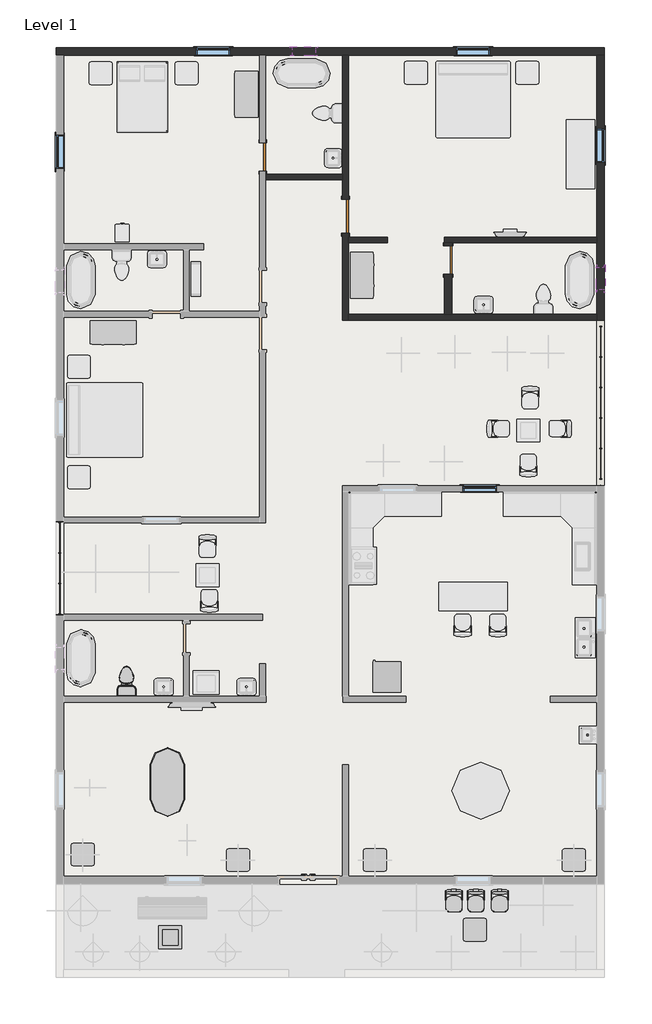
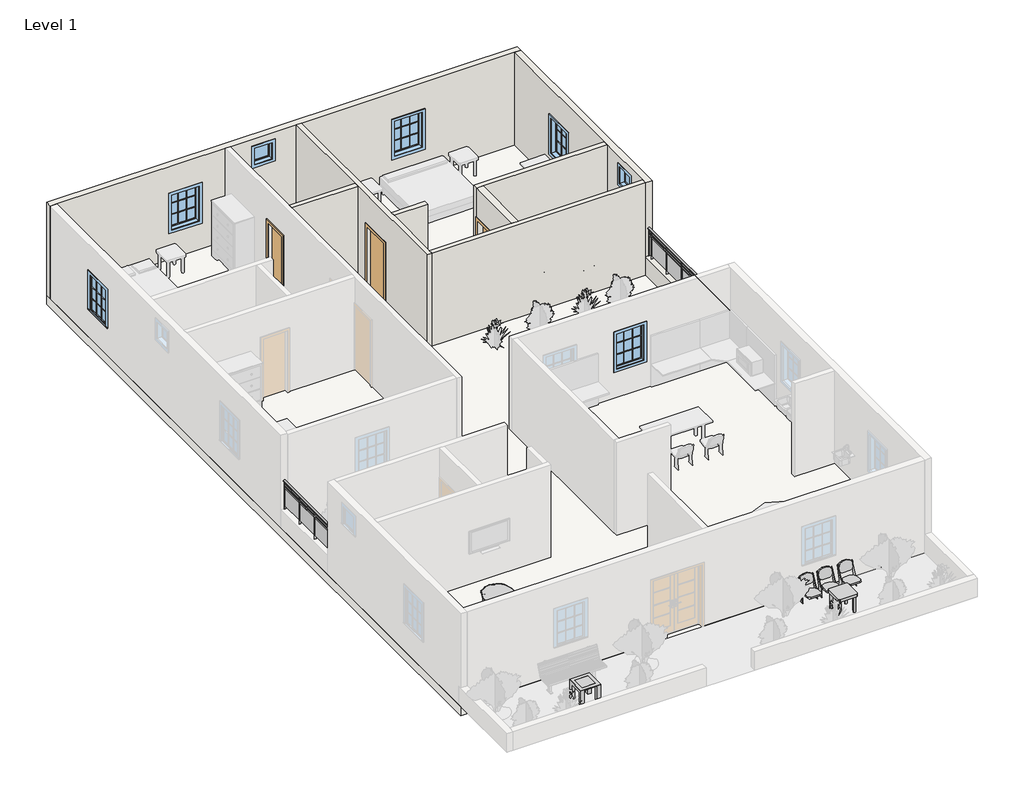
# One storey, part 2 of 3: 10 furniture elements, 9 walls, 7 windows, 3 doors, 2 flow terminals, 2 railings, 1 slab.
"""IFC4 building model written with IfcOpenShell, lengths in millimetres."""

from ifc_helpers import new_model, si_unit, point, frame, origin, origin_with_axes, place, context, project, spatial, polyline, ellipse_curve, trimmed, outline, extrude, faceted_brep, transform, mapped, element, save
from ifc_brep_helpers import plane_surface, extruded_surface, advanced_brep
from components import door_059fdd7e, door_53b1b562, door_193fcfdc, flow_terminal_accce45a, toilet_domestic_3d_toilet_domestic_3d_f7549cf7, toilet_domestic_3d_toilet_domestic_3d_183bbd19, furniture_3d1d9cbc, furniture_b5c51a22, furniture_2c34a4f9, furniture_31d08a24, window_29c06734, window_5c190c7e, window_e41d21a6

model = new_model("IFC4")

# Units and contexts
model_context = context("Model", 3, world=origin())
ifc_project = project(units=[si_unit("LENGTHUNIT", "METRE", prefix="MILLI")], contexts=[model_context])

# Site, building, storey
site = spatial("IfcSite", under=ifc_project)
building = spatial("IfcBuilding", under=site)
storey = spatial("IfcBuildingStorey", under=building, Name="Level 1", Elevation=0.0)

# Doors
placement = place(None, origin())
door_shape = door_059fdd7e(model_context)
element("IfcDoor", 1, ObjectType="Single-Flush : 30\" x 80\"", at=placement, inside=storey, context=model_context, shape_type="MappedRepresentation", body=[
    mapped(door_shape, transform((-9555.9446525, 9738.3002171, 0.0), x_axis=(0.0, -1.0, 0.0), y_axis=(1.0, 0.0, 0.0), z_axis=(0.0, 0.0, 1.0))),
])
door_2_shape = door_53b1b562(model_context)
element("IfcDoor", 2, ObjectType="Single-Flush : 30\" x 80\"", at=placement, inside=storey, context=model_context, shape_type="MappedRepresentation", body=[
    mapped(door_2_shape, transform((-4602.9446525, 6995.1002171, 0.0), x_axis=(0.0, 1.0, 0.0), y_axis=(-1.0, 0.0, 0.0), z_axis=(0.0, 0.0, 1.0))),
])
door_3_shape = door_193fcfdc(model_context)
element("IfcDoor", 3, ObjectType="Single-Flush : 36\" x 80\"", at=placement, inside=storey, context=model_context, shape_type="MappedRepresentation", body=[
    mapped(door_3_shape, transform((-7346.1446525, 8163.5002171, 0.0), x_axis=(0.0, -1.0, 0.0), y_axis=(1.0, 0.0, 0.0), z_axis=(0.0, 0.0, 1.0))),
])

# Flow terminals
flow_terminal_shape = flow_terminal_accce45a(model_context)
element("IfcFlowTerminal", 4, ObjectType="Floor Drain - Round : 5\" Strainer - 2\" Drain", at=placement, inside=storey, context=model_context, shape_type="MappedRepresentation", body=[
    mapped(flow_terminal_shape, transform((-13721.5446525, -4257.0997829, 0.0), x_axis=(1.0, 0.0, 0.0), y_axis=(0.0, 1.0, 0.0), z_axis=(0.0, 0.0, 1.0))),
])
toilet_domestic_3d_toilet_domestic_3d_shape = toilet_domestic_3d_toilet_domestic_3d_f7549cf7(model_context)
toilet_domestic_3d_toilet_domestic_3d_2_shape = toilet_domestic_3d_toilet_domestic_3d_183bbd19(model_context)
element("IfcFlowTerminal", 5, ObjectType="Toilet-Domestic-3D : Toilet-Domestic-3D", at=placement, inside=storey, context=model_context, shape_type="MappedRepresentation", body=[
    mapped(toilet_domestic_3d_toilet_domestic_3d_shape, transform((-13188.1446525, -4143.4037556, 0.0), x_axis=(-1.0000000000000004, 0.0, 0.0), y_axis=(0.0, -1.0000000000000004, 0.0), z_axis=(0.0, 0.0, 1.0))),
    mapped(toilet_domestic_3d_toilet_domestic_3d_2_shape, transform((-13188.1446525, -4143.4037556, 0.0), x_axis=(-1.0000000000000004, 0.0, 0.0), y_axis=(0.0, -1.0000000000000004, 0.0), z_axis=(0.0, 0.0, 1.0))),
])

# Furniture
furniture_shape = furniture_3d1d9cbc(model_context)
element("IfcFurniture", 6, ObjectType="Seating-Auditorium : 18\" x 24\" x 30\"", at=placement, inside=storey, context=model_context, shape_type="MappedRepresentation", body=[
    mapped(furniture_shape, transform((-4289.8167836, -9883.8243731, 0.0), x_axis=(-1.0000000000000004, 0.0, 0.0), y_axis=(0.0, -1.0000000000000004, 0.0), z_axis=(0.0, 0.0, 1.0))),
])
element("IfcFurniture", 7, ObjectType="Seating-Auditorium : 18\" x 24\" x 30\"", at=placement, inside=storey, context=model_context, shape_type="MappedRepresentation", body=[
    mapped(furniture_shape, transform((-3705.6167836, -9883.8243731, 0.0), x_axis=(-1.0000000000000004, 0.0, 0.0), y_axis=(0.0, -1.0000000000000004, 0.0), z_axis=(0.0, 0.0, 1.0))),
])
element("IfcFurniture", 8, ObjectType="Seating-Auditorium : 18\" x 24\" x 30\"", at=placement, inside=storey, context=model_context, shape_type="MappedRepresentation", body=[
    mapped(furniture_shape, transform((-3070.6167836, -9883.8243731, 0.0), x_axis=(-1.0000000000000004, 0.0, 0.0), y_axis=(0.0, -1.0000000000000004, 0.0), z_axis=(0.0, 0.0, 1.0))),
])
furniture_2_shape = furniture_b5c51a22(model_context)
element("IfcFurniture", 9, ObjectType="Table-Coffee : 24\" x 24\" x 24\"", at=placement, inside=storey, context=model_context, shape_type="MappedRepresentation", body=[
    mapped(furniture_2_shape, transform((-12038.0104192, -11159.5108607, 0.0), x_axis=(1.0, 0.0, 0.0), y_axis=(0.0, 1.0, 0.0), z_axis=(0.0, 0.0, 1.0))),
])
furniture_3_shape = furniture_2c34a4f9(model_context)
element("IfcFurniture", 10, ObjectType="Table-Dining Oval : 36\" x 72\"", at=placement, inside=storey, context=model_context, shape_type="MappedRepresentation", body=[
    mapped(furniture_3_shape, transform((-12454.0430131, -6522.2801108, 0.0), x_axis=(0.0, 1.0000000000000002, 0.0), y_axis=(-1.0000000000000002, 0.0, 0.0), z_axis=(0.0, 0.0, 1.0))),
])
furniture_4_shape = furniture_31d08a24(model_context)
element("IfcFurniture", 11, ObjectType="Table-End : 24\" x 24\"", at=placement, inside=storey, context=model_context, shape_type="MappedRepresentation", body=[
    mapped(furniture_4_shape, transform((-14665.0782828, -9006.8997829, 0.0), x_axis=(1.0, 0.0, 0.0), y_axis=(0.0, 1.0, 0.0), z_axis=(0.0, 0.0, 1.0))),
])
element("IfcFurniture", 12, ObjectType="Table-End : 24\" x 24\"", at=placement, inside=storey, context=model_context, shape_type="MappedRepresentation", body=[
    mapped(furniture_4_shape, transform((-10524.8782828, -9152.9497829, 0.0), x_axis=(1.0, 0.0, 0.0), y_axis=(0.0, 1.0, 0.0), z_axis=(0.0, 0.0, 1.0))),
])
element("IfcFurniture", 13, ObjectType="Table-End : 24\" x 24\"", at=placement, inside=storey, context=model_context, shape_type="MappedRepresentation", body=[
    mapped(furniture_4_shape, transform((-6867.2782828, -9152.9497829, 0.0), x_axis=(1.0, 0.0, 0.0), y_axis=(0.0, 1.0, 0.0), z_axis=(0.0, 0.0, 1.0))),
])
element("IfcFurniture", 14, ObjectType="Table-End : 24\" x 24\"", at=placement, inside=storey, context=model_context, shape_type="MappedRepresentation", body=[
    mapped(furniture_4_shape, transform((-1558.6782828, -9152.9497829, 0.0), x_axis=(1.0, 0.0, 0.0), y_axis=(0.0, 1.0, 0.0), z_axis=(0.0, 0.0, 1.0))),
])
element("IfcFurniture", 15, ObjectType="Table-End : 24\" x 24\"", at=placement, inside=storey, context=model_context, shape_type="MappedRepresentation", body=[
    mapped(furniture_4_shape, transform((-4200.2782828, -11013.4997829, 0.0), x_axis=(1.0, 0.0, 0.0), y_axis=(0.0, 1.0, 0.0), z_axis=(0.0, 0.0, 1.0))),
])

# Railings
element("IfcRailing", 16, ObjectType="Glass Panel - Bottom Fill", at=placement, inside=storey, context=model_context, shape_type="SolidModel", body=[
    advanced_brep(
    [(-14928.0446525, 35.5002171, 1524.0), (-15004.2446525, 35.5002171, 1524.0), (-14928.0446525, -2479.0997829, 1524.0), (-15004.2446525, -2479.0997829, 1524.0)],
    [
        (0, 1, ellipse_curve(frame((-14966.1446525, 35.5002171, 1524.0), z_axis=(0.0, 1.0, 0.0), x_axis=(-1.0, 0.0, 0.0)), 38.1, 28.575)),
        (1, 0, ellipse_curve(frame((-14966.1446525, 35.5002171, 1524.0), z_axis=(0.0, 1.0, 0.0), x_axis=(-1.0, 0.0, 0.0)), 38.1, 28.575)),
        (2, 3, ellipse_curve(frame((-14966.1446525, -2479.0997829, 1524.0), z_axis=(0.0, -1.0, 0.0), x_axis=(-1.0, 0.0, 0.0)), 38.1, 28.575)),
        (3, 2, ellipse_curve(frame((-14966.1446525, -2479.0997829, 1524.0), z_axis=(0.0, -1.0, 0.0), x_axis=(-1.0, 0.0, 0.0)), 38.1, 28.575)),
        (0, 2),
        (3, 1),
    ],
    [
        plane_surface(frame((-14966.1446525, 35.5002171, 1524.0), z_axis=(0.0, 1.0, 0.0), x_axis=(0.0, 0.0, -1.0))),
        plane_surface(frame((-14966.1446525, -2479.0997829, 1524.0), z_axis=(0.0, -1.0, 0.0), x_axis=(0.0, 0.0, -1.0))),
        extruded_surface(trimmed(ellipse_curve(frame((-14966.1446525, -2479.0997829, 1524.0), z_axis=(0.0, 1.0, 0.0), x_axis=(-1.0, 0.0, 0.0)), 38.1, 28.575), [point((-14928.0446525, -2479.0997829, 1524.0))], [point((-15004.2446525, -2479.0997829, 1524.0))], True, "CARTESIAN"), (0.0, 2514.6, 0.0), 2514.6),
        extruded_surface(trimmed(ellipse_curve(frame((-14966.1446525, -2479.0997829, 1524.0), z_axis=(0.0, 1.0, 0.0), x_axis=(-1.0, 0.0, 0.0)), 38.1, 28.575), [point((-15004.2446525, -2479.0997829, 1524.0))], [point((-14928.0446525, -2479.0997829, 1524.0))], True, "CARTESIAN"), (0.0, 2514.6, 0.0), 2514.6),
    ],
    [
        (0, [[1, 2]]),
        (1, [[3, 4]]),
        (2, [[-1, 5, -4, 6]]),
        (3, [[-2, -6, -3, -5]]),
    ],
),
    extrude(outline(polyline([(-14978.8446525, 35.5002171), (-14953.4446525, 35.5002171), (-14953.4446525, -2479.0997829), (-14978.8446525, -2479.0997829), (-14978.8446525, 35.5002171)])), frame((0.0, 0.0, 1409.7), z_axis=(0.0, 0.0, 1.0), x_axis=(1.0, 0.0, 0.0)), (0.0, 0.0, 1.0), 25.4),
    extrude(outline(polyline([(-14978.8446525, 35.5002171), (-14953.4446525, 35.5002171), (-14953.4446525, -2479.0997829), (-14978.8446525, -2479.0997829), (-14978.8446525, 35.5002171)])), frame((0.0, 0.0, 1308.1), z_axis=(0.0, 0.0, 1.0), x_axis=(1.0, 0.0, 0.0)), (0.0, 0.0, 1.0), 25.4),
    extrude(outline(polyline([(-14991.5446525, -2434.6497829), (-14940.7446525, -2434.6497829), (-14940.7446525, -2447.3497829), (-14991.5446525, -2447.3497829), (-14991.5446525, -2434.6497829)])), frame((0.0, 0.0, 609.6), z_axis=(0.0, 0.0, 1.0), x_axis=(1.0, 0.0, 0.0)), (0.0, 0.0, 1.0), 885.6788223),
    extrude(outline(polyline([(-14959.6094955, -1628.1997829), (-14959.6094955, -2440.9997829), (-14965.9594955, -2440.9997829), (-14965.9594955, -1628.1997829), (-14959.6094955, -1628.1997829)])), frame((0.0, 0.0, 711.2), z_axis=(0.0, 0.0, 1.0), x_axis=(1.0, 0.0, 0.0)), (0.0, 0.0, 1.0), 596.9),
    extrude(outline(polyline([(-14991.5446525, -1621.8497829), (-14940.7446525, -1621.8497829), (-14940.7446525, -1634.5497829), (-14991.5446525, -1634.5497829), (-14991.5446525, -1621.8497829)])), frame((0.0, 0.0, 609.6), z_axis=(0.0, 0.0, 1.0), x_axis=(1.0, 0.0, 0.0)), (0.0, 0.0, 1.0), 885.6788223),
    extrude(outline(polyline([(-14959.6094955, -815.3997829), (-14959.6094955, -1628.1997829), (-14965.9594955, -1628.1997829), (-14965.9594955, -815.3997829), (-14959.6094955, -815.3997829)])), frame((0.0, 0.0, 711.2), z_axis=(0.0, 0.0, 1.0), x_axis=(1.0, 0.0, 0.0)), (0.0, 0.0, 1.0), 596.9),
    extrude(outline(polyline([(-14991.5446525, -809.0497829), (-14940.7446525, -809.0497829), (-14940.7446525, -821.7497829), (-14991.5446525, -821.7497829), (-14991.5446525, -809.0497829)])), frame((0.0, 0.0, 609.6), z_axis=(0.0, 0.0, 1.0), x_axis=(1.0, 0.0, 0.0)), (0.0, 0.0, 1.0), 885.6788223),
    extrude(outline(polyline([(-14959.6094955, -2.5997829), (-14959.6094955, -815.3997829), (-14965.9594955, -815.3997829), (-14965.9594955, -2.5997829), (-14959.6094955, -2.5997829)])), frame((0.0, 0.0, 711.2), z_axis=(0.0, 0.0, 1.0), x_axis=(1.0, 0.0, 0.0)), (0.0, 0.0, 1.0), 596.9),
    extrude(outline(polyline([(-14991.5446525, 3.7502171), (-14940.7446525, 3.7502171), (-14940.7446525, -8.9497829), (-14991.5446525, -8.9497829), (-14991.5446525, 3.7502171)])), frame((0.0, 0.0, 609.6), z_axis=(0.0, 0.0, 1.0), x_axis=(1.0, 0.0, 0.0)), (0.0, 0.0, 1.0), 885.6788223),
    extrude(outline(polyline([(-14975.6696525, -2466.3997829), (-14956.6196525, -2466.3997829), (-14956.6196525, -2485.4497829), (-14975.6696525, -2485.4497829), (-14975.6696525, -2466.3997829)])), frame((0.0, 0.0, 609.6), z_axis=(0.0, 0.0, 1.0), x_axis=(1.0, 0.0, 0.0)), (0.0, 0.0, 1.0), 885.6788223),
    extrude(outline(polyline([(-14975.6696525, 41.8502171), (-14956.6196525, 41.8502171), (-14956.6196525, 22.8002171), (-14975.6696525, 22.8002171), (-14975.6696525, 41.8502171)])), frame((0.0, 0.0, 609.6), z_axis=(0.0, 0.0, 1.0), x_axis=(1.0, 0.0, 0.0)), (0.0, 0.0, 1.0), 885.6788223),
])
element("IfcRailing", 17, ObjectType="Glass Panel - Bottom Fill", at=placement, inside=storey, context=model_context, shape_type="SolidModel", body=[
    advanced_brep(
    [(-500.8446525, 5394.9002171, 1524.0), (-577.0446525, 5394.9002171, 1524.0), (-500.8446525, 975.3002171, 1524.0), (-577.0446525, 975.3002171, 1524.0)],
    [
        (0, 1, ellipse_curve(frame((-538.9446525, 5394.9002171, 1524.0), z_axis=(0.0, 1.0, 0.0), x_axis=(-1.0, 0.0, 0.0)), 38.1, 28.575)),
        (1, 0, ellipse_curve(frame((-538.9446525, 5394.9002171, 1524.0), z_axis=(0.0, 1.0, 0.0), x_axis=(-1.0, 0.0, 0.0)), 38.1, 28.575)),
        (2, 3, ellipse_curve(frame((-538.9446525, 975.3002171, 1524.0), z_axis=(0.0, -1.0, 0.0), x_axis=(-1.0, 0.0, 0.0)), 38.1, 28.575)),
        (3, 2, ellipse_curve(frame((-538.9446525, 975.3002171, 1524.0), z_axis=(0.0, -1.0, 0.0), x_axis=(-1.0, 0.0, 0.0)), 38.1, 28.575)),
        (0, 2),
        (3, 1),
    ],
    [
        plane_surface(frame((-538.9446525, 5394.9002171, 1524.0), z_axis=(0.0, 1.0, 0.0), x_axis=(0.0, 0.0, -1.0))),
        plane_surface(frame((-538.9446525, 975.3002171, 1524.0), z_axis=(0.0, -1.0, 0.0), x_axis=(0.0, 0.0, -1.0))),
        extruded_surface(trimmed(ellipse_curve(frame((-538.9446525, 975.3002171, 1524.0), z_axis=(0.0, 1.0, 0.0), x_axis=(-1.0, 0.0, 0.0)), 38.1, 28.575), [point((-500.8446525, 975.3002171, 1524.0))], [point((-577.0446525, 975.3002171, 1524.0))], True, "CARTESIAN"), (0.0, 4419.6, 0.0), 4419.6),
        extruded_surface(trimmed(ellipse_curve(frame((-538.9446525, 975.3002171, 1524.0), z_axis=(0.0, 1.0, 0.0), x_axis=(-1.0, 0.0, 0.0)), 38.1, 28.575), [point((-577.0446525, 975.3002171, 1524.0))], [point((-500.8446525, 975.3002171, 1524.0))], True, "CARTESIAN"), (0.0, 4419.6, 0.0), 4419.6),
    ],
    [
        (0, [[1, 2]]),
        (1, [[3, 4]]),
        (2, [[-1, 5, -4, 6]]),
        (3, [[-2, -6, -3, -5]]),
    ],
),
    extrude(outline(polyline([(-551.6446525, 5394.9002171), (-526.2446525, 5394.9002171), (-526.2446525, 975.3002171), (-551.6446525, 975.3002171), (-551.6446525, 5394.9002171)])), frame((0.0, 0.0, 1409.7), z_axis=(0.0, 0.0, 1.0), x_axis=(1.0, 0.0, 0.0)), (0.0, 0.0, 1.0), 25.4),
    extrude(outline(polyline([(-551.6446525, 5394.9002171), (-526.2446525, 5394.9002171), (-526.2446525, 975.3002171), (-551.6446525, 975.3002171), (-551.6446525, 5394.9002171)])), frame((0.0, 0.0, 1308.1), z_axis=(0.0, 0.0, 1.0), x_axis=(1.0, 0.0, 0.0)), (0.0, 0.0, 1.0), 25.4),
    extrude(outline(polyline([(-564.3446525, 1159.4502171), (-513.5446525, 1159.4502171), (-513.5446525, 1146.7502171), (-564.3446525, 1146.7502171), (-564.3446525, 1159.4502171)])), frame((0.0, 0.0, 609.6), z_axis=(0.0, 0.0, 1.0), x_axis=(1.0, 0.0, 0.0)), (0.0, 0.0, 1.0), 885.6788223),
    extrude(outline(polyline([(-532.4094955, 1965.9002171), (-532.4094955, 1153.1002171), (-538.7594955, 1153.1002171), (-538.7594955, 1965.9002171), (-532.4094955, 1965.9002171)])), frame((0.0, 0.0, 711.2), z_axis=(0.0, 0.0, 1.0), x_axis=(1.0, 0.0, 0.0)), (0.0, 0.0, 1.0), 596.9),
    extrude(outline(polyline([(-564.3446525, 1972.2502171), (-513.5446525, 1972.2502171), (-513.5446525, 1959.5502171), (-564.3446525, 1959.5502171), (-564.3446525, 1972.2502171)])), frame((0.0, 0.0, 609.6), z_axis=(0.0, 0.0, 1.0), x_axis=(1.0, 0.0, 0.0)), (0.0, 0.0, 1.0), 885.6788223),
    extrude(outline(polyline([(-532.4094955, 2778.7002171), (-532.4094955, 1965.9002171), (-538.7594955, 1965.9002171), (-538.7594955, 2778.7002171), (-532.4094955, 2778.7002171)])), frame((0.0, 0.0, 711.2), z_axis=(0.0, 0.0, 1.0), x_axis=(1.0, 0.0, 0.0)), (0.0, 0.0, 1.0), 596.9),
    extrude(outline(polyline([(-564.3446525, 2785.0502171), (-513.5446525, 2785.0502171), (-513.5446525, 2772.3502171), (-564.3446525, 2772.3502171), (-564.3446525, 2785.0502171)])), frame((0.0, 0.0, 609.6), z_axis=(0.0, 0.0, 1.0), x_axis=(1.0, 0.0, 0.0)), (0.0, 0.0, 1.0), 885.6788223),
    extrude(outline(polyline([(-532.4094955, 3591.5002171), (-532.4094955, 2778.7002171), (-538.7594955, 2778.7002171), (-538.7594955, 3591.5002171), (-532.4094955, 3591.5002171)])), frame((0.0, 0.0, 711.2), z_axis=(0.0, 0.0, 1.0), x_axis=(1.0, 0.0, 0.0)), (0.0, 0.0, 1.0), 596.9),
    extrude(outline(polyline([(-564.3446525, 3597.8502171), (-513.5446525, 3597.8502171), (-513.5446525, 3585.1502171), (-564.3446525, 3585.1502171), (-564.3446525, 3597.8502171)])), frame((0.0, 0.0, 609.6), z_axis=(0.0, 0.0, 1.0), x_axis=(1.0, 0.0, 0.0)), (0.0, 0.0, 1.0), 885.6788223),
    extrude(outline(polyline([(-532.4094955, 4404.3002171), (-532.4094955, 3591.5002171), (-538.7594955, 3591.5002171), (-538.7594955, 4404.3002171), (-532.4094955, 4404.3002171)])), frame((0.0, 0.0, 711.2), z_axis=(0.0, 0.0, 1.0), x_axis=(1.0, 0.0, 0.0)), (0.0, 0.0, 1.0), 596.9),
    extrude(outline(polyline([(-564.3446525, 4410.6502171), (-513.5446525, 4410.6502171), (-513.5446525, 4397.9502171), (-564.3446525, 4397.9502171), (-564.3446525, 4410.6502171)])), frame((0.0, 0.0, 609.6), z_axis=(0.0, 0.0, 1.0), x_axis=(1.0, 0.0, 0.0)), (0.0, 0.0, 1.0), 885.6788223),
    extrude(outline(polyline([(-532.4094955, 5217.1002171), (-532.4094955, 4404.3002171), (-538.7594955, 4404.3002171), (-538.7594955, 5217.1002171), (-532.4094955, 5217.1002171)])), frame((0.0, 0.0, 711.2), z_axis=(0.0, 0.0, 1.0), x_axis=(1.0, 0.0, 0.0)), (0.0, 0.0, 1.0), 596.9),
    extrude(outline(polyline([(-564.3446525, 5223.4502171), (-513.5446525, 5223.4502171), (-513.5446525, 5210.7502171), (-564.3446525, 5210.7502171), (-564.3446525, 5223.4502171)])), frame((0.0, 0.0, 609.6), z_axis=(0.0, 0.0, 1.0), x_axis=(1.0, 0.0, 0.0)), (0.0, 0.0, 1.0), 885.6788223),
    extrude(outline(polyline([(-548.4696525, 988.0002171), (-529.4196525, 988.0002171), (-529.4196525, 968.9502171), (-548.4696525, 968.9502171), (-548.4696525, 988.0002171)])), frame((0.0, 0.0, 609.6), z_axis=(0.0, 0.0, 1.0), x_axis=(1.0, 0.0, 0.0)), (0.0, 0.0, 1.0), 885.6788223),
    extrude(outline(polyline([(-548.4696525, 5401.2502171), (-529.4196525, 5401.2502171), (-529.4196525, 5382.2002171), (-548.4696525, 5382.2002171), (-548.4696525, 5401.2502171)])), frame((0.0, 0.0, 609.6), z_axis=(0.0, 0.0, 1.0), x_axis=(1.0, 0.0, 0.0)), (0.0, 0.0, 1.0), 885.6788223),
])

# Slab
element("IfcSlab", 18, ObjectType="Generic - 12\"", at=placement, inside=storey, context=model_context, shape_type="SweptSolid", body=[
    extrude(outline(polyline([(-437.3446525, 12659.3002171), (-437.3446525, -9641.8997829), (-15067.7446525, -9641.8997829), (-15067.7446525, 12659.3002171), (-437.3446525, 12659.3002171)])), frame((0.0, 0.0, -304.8), z_axis=(0.0, 0.0, 1.0), x_axis=(1.0, 0.0, 0.0)), (0.0, 0.0, 1.0), 304.8),
])

# Walls
element("IfcWall", 19, ObjectType="Generic - 2'", at=placement, inside=storey, context=model_context, shape_type="Brep", body=[
    faceted_brep([(-640.5446525, 5471.1002171, 0.0), (-640.5446525, 5394.9002171, 0.0), (-640.5446525, 975.3002171, 0.0), (-640.5446525, 899.1002171, 0.0), (-640.5446525, 899.1002171, 609.6), (-640.5446525, 5471.1002171, 609.6), (-437.3446525, 5471.1002171, 0.0), (-437.3446525, 5471.1002171, 609.6), (-437.3446525, 899.1002171, 609.6), (-437.3446525, 899.1002171, 0.0)], [[[0, 1, 2, 3, 4, 5]], [[6, 7, 8, 9]], [[3, 2, 1, 0, 6, 9]], [[4, 3, 9, 8]], [[5, 4, 8, 7]], [[0, 5, 7, 6]]]),
])
element("IfcWall", 20, ObjectType="Generic - 8\"", at=placement, inside=storey, context=model_context, shape_type="Brep", body=[
    faceted_brep([(-15067.7446525, 12456.1002171, 0.0), (-14864.5446525, 12456.1002171, 0.0), (-9632.1446525, 12456.1002171, 0.0), (-9479.7446525, 12456.1002171, 0.0), (-7422.3446525, 12456.1002171, 0.0), (-7269.9446525, 12456.1002171, 0.0), (-640.5446525, 12456.1002171, 0.0), (-437.3446525, 12456.1002171, 0.0), (-437.3446525, 12456.1002171, 3048.0), (-640.5446525, 12456.1002171, 3048.0), (-7269.9446525, 12456.1002171, 3048.0), (-7422.3446525, 12456.1002171, 3048.0), (-9479.7446525, 12456.1002171, 3048.0), (-9632.1446525, 12456.1002171, 3048.0), (-14864.5446525, 12456.1002171, 3048.0), (-15067.7446525, 12456.1002171, 3048.0), (-3485.3446525, 12456.1002171, 2133.6), (-3485.3446525, 12456.1002171, 914.4), (-4399.7446525, 12456.1002171, 914.4), (-4399.7446525, 12456.1002171, 2133.6), (-10419.5446525, 12456.1002171, 2133.6), (-10419.5446525, 12456.1002171, 914.4), (-11333.9446525, 12456.1002171, 914.4), (-11333.9446525, 12456.1002171, 2133.6), (-8146.2446525, 12456.1002171, 2768.6), (-8146.2446525, 12456.1002171, 2159.0), (-8755.8446525, 12456.1002171, 2159.0), (-8755.8446525, 12456.1002171, 2768.6), (-15067.7446525, 12659.3002171, 0.0), (-15067.7446525, 12659.3002171, 3048.0), (-437.3446525, 12659.3002171, 3048.0), (-437.3446525, 12659.3002171, 0.0), (-3485.3446525, 12659.3002171, 2133.6), (-4399.7446525, 12659.3002171, 2133.6), (-4399.7446525, 12659.3002171, 914.4), (-3485.3446525, 12659.3002171, 914.4), (-10419.5446525, 12659.3002171, 2133.6), (-11333.9446525, 12659.3002171, 2133.6), (-11333.9446525, 12659.3002171, 914.4), (-10419.5446525, 12659.3002171, 914.4), (-8146.2446525, 12659.3002171, 2768.6), (-8755.8446525, 12659.3002171, 2768.6), (-8755.8446525, 12659.3002171, 2159.0), (-8146.2446525, 12659.3002171, 2159.0)], [[[0, 1, 2, 3, 4, 5, 6, 7, 8, 9, 10, 11, 12, 13, 14, 15], [16, 17, 18, 19], [20, 21, 22, 23], [24, 25, 26, 27]], [[28, 29, 30, 31], [32, 33, 34, 35], [36, 37, 38, 39], [40, 41, 42, 43]], [[7, 6, 5, 4, 3, 2, 1, 0, 28, 31]], [[8, 7, 31, 30]], [[0, 15, 29, 28]], [[17, 16, 32, 35]], [[18, 17, 35, 34]], [[19, 18, 34, 33]], [[16, 19, 33, 32]], [[21, 20, 36, 39]], [[22, 21, 39, 38]], [[23, 22, 38, 37]], [[20, 23, 37, 36]], [[25, 24, 40, 43]], [[26, 25, 43, 42]], [[27, 26, 42, 41]], [[24, 27, 41, 40]], [[15, 14, 13, 12, 11, 10, 9, 8, 30, 29]]]),
])
element("IfcWall", 21, ObjectType="Generic - 8\"", at=placement, inside=storey, context=model_context, shape_type="Brep", body=[
    faceted_brep([(-640.5446525, 12456.1002171, 0.0), (-640.5446525, 7604.7002171, 0.0), (-640.5446525, 7452.3002171, 0.0), (-640.5446525, 5547.3002171, 0.0), (-640.5446525, 5471.1002171, 0.0), (-640.5446525, 5471.1002171, 609.6), (-640.5446525, 5394.9002171, 609.6), (-640.5446525, 5394.9002171, 3048.0), (-640.5446525, 5547.3002171, 3048.0), (-640.5446525, 7452.3002171, 3048.0), (-640.5446525, 7604.7002171, 3048.0), (-640.5446525, 12456.1002171, 3048.0), (-640.5446525, 9585.9002171, 2133.6), (-640.5446525, 9585.9002171, 914.4), (-640.5446525, 10500.3002171, 914.4), (-640.5446525, 10500.3002171, 2133.6), (-640.5446525, 6195.0002171, 2768.6), (-640.5446525, 6195.0002171, 2159.0), (-640.5446525, 6804.6002171, 2159.0), (-640.5446525, 6804.6002171, 2768.6), (-437.3446525, 12456.1002171, 0.0), (-437.3446525, 12456.1002171, 3048.0), (-437.3446525, 5394.9002171, 3048.0), (-437.3446525, 5394.9002171, 609.6), (-437.3446525, 5471.1002171, 609.6), (-437.3446525, 5471.1002171, 0.0), (-437.3446525, 9585.9002171, 2133.6), (-437.3446525, 10500.3002171, 2133.6), (-437.3446525, 10500.3002171, 914.4), (-437.3446525, 9585.9002171, 914.4), (-437.3446525, 6195.0002171, 2768.6), (-437.3446525, 6804.6002171, 2768.6), (-437.3446525, 6804.6002171, 2159.0), (-437.3446525, 6195.0002171, 2159.0)], [[[0, 1, 2, 3, 4, 5, 6, 7, 8, 9, 10, 11], [12, 13, 14, 15], [16, 17, 18, 19]], [[20, 21, 22, 23, 24, 25], [26, 27, 28, 29], [30, 31, 32, 33]], [[4, 3, 2, 1, 0, 20, 25]], [[0, 11, 21, 20]], [[13, 12, 26, 29]], [[14, 13, 29, 28]], [[15, 14, 28, 27]], [[12, 15, 27, 26]], [[17, 16, 30, 33]], [[18, 17, 33, 32]], [[19, 18, 32, 31]], [[16, 19, 31, 30]], [[5, 4, 25, 24]], [[23, 6, 5, 24]], [[7, 6, 23, 22]], [[11, 10, 9, 8, 7, 22, 21]]]),
])
element("IfcWall", 22, ObjectType="Generic - 8\"", at=placement, inside=storey, context=model_context, shape_type="SweptSolid", body=[
    extrude(outline(polyline([(7452.3002171, 0.0), (7376.1002171, 0.0), (7376.1002171, 2032.0), (6614.1002171, 2032.0), (6614.1002171, 0.0), (5547.3002171, 0.0), (5547.3002171, 3048.0), (7452.3002171, 3048.0), (7452.3002171, 0.0)])), frame((-4704.5446525, 0.0, 0.0), z_axis=(1.0, 0.0, 0.0), x_axis=(0.0, 1.0, 0.0)), (0.0, 0.0, 1.0), 203.2),
])
element("IfcWall", 23, ObjectType="INNER 6\"", at=placement, inside=storey, context=model_context, shape_type="Brep", body=[
    faceted_brep([(-7422.3446525, 7706.3002171, 2032.0), (-7422.3446525, 7706.3002171, 0.0), (-7422.3446525, 5394.9002171, 0.0), (-7422.3446525, 5394.9002171, 3048.0), (-7422.3446525, 9128.7002171, 3048.0), (-7422.3446525, 9281.1002171, 3048.0), (-7422.3446525, 12456.1002171, 3048.0), (-7422.3446525, 12456.1002171, 0.0), (-7422.3446525, 9281.1002171, 0.0), (-7422.3446525, 9128.7002171, 0.0), (-7422.3446525, 8620.7002171, 0.0), (-7422.3446525, 8620.7002171, 2032.0), (-7269.9446525, 5394.9002171, 0.0), (-7269.9446525, 5547.3002171, 0.0), (-7269.9446525, 7452.3002171, 0.0), (-7269.9446525, 7604.7002171, 0.0), (-7269.9446525, 7706.3002171, 0.0), (-7269.9446525, 7706.3002171, 2032.0), (-7269.9446525, 8620.7002171, 2032.0), (-7269.9446525, 8620.7002171, 0.0), (-7269.9446525, 12456.1002171, 0.0), (-7269.9446525, 12456.1002171, 3048.0), (-7269.9446525, 7604.7002171, 3048.0), (-7269.9446525, 7452.3002171, 3048.0), (-7269.9446525, 5547.3002171, 3048.0), (-7269.9446525, 5394.9002171, 3048.0)], [[[0, 1, 2, 3, 4, 5, 6, 7, 8, 9, 10, 11]], [[12, 13, 14, 15, 16, 17, 18, 19, 20, 21, 22, 23, 24, 25]], [[2, 1, 16, 15, 14, 13, 12]], [[10, 9, 8, 7, 20, 19]], [[7, 6, 21, 20]], [[3, 2, 12, 25]], [[17, 16, 1, 0]], [[18, 17, 0, 11]], [[19, 18, 11, 10]], [[6, 5, 4, 3, 25, 24, 23, 22, 21]]]),
])
element("IfcWall", 24, ObjectType="INNER 6\"", at=placement, inside=storey, context=model_context, shape_type="SweptSolid", body=[
    extrude(outline(polyline([(-7422.3446525, 9128.7002171), (-9479.7446525, 9128.7002171), (-9479.7446525, 9281.1002171), (-7422.3446525, 9281.1002171), (-7422.3446525, 9128.7002171)])), origin_with_axes(), (0.0, 0.0, 1.0), 3048.0),
])
element("IfcWall", 25, ObjectType="INNER 6\"", at=placement, inside=storey, context=model_context, shape_type="Brep", body=[
    faceted_brep([(-7269.9446525, 5394.9002171, 0.0), (-640.5446525, 5394.9002171, 0.0), (-640.5446525, 5394.9002171, 609.6), (-640.5446525, 5394.9002171, 3048.0), (-7269.9446525, 5394.9002171, 3048.0), (-7269.9446525, 5547.3002171, 0.0), (-7269.9446525, 5547.3002171, 3048.0), (-4704.5446525, 5547.3002171, 3048.0), (-4501.3446525, 5547.3002171, 3048.0), (-640.5446525, 5547.3002171, 3048.0), (-640.5446525, 5547.3002171, 0.0), (-4501.3446525, 5547.3002171, 0.0), (-4704.5446525, 5547.3002171, 0.0), (-640.5446525, 5471.1002171, 0.0)], [[[0, 1, 2, 3, 4]], [[5, 6, 7, 8, 9, 10, 11, 12]], [[1, 0, 5, 12, 11, 10, 13]], [[0, 4, 6, 5]], [[1, 13, 10, 9, 3, 2]], [[4, 3, 9, 8, 7, 6]]]),
])
element("IfcWall", 26, ObjectType="INNER 6\"", at=placement, inside=storey, context=model_context, shape_type="SweptSolid", body=[
    extrude(outline(polyline([(-6228.5446525, 7452.3002171), (-7269.9446525, 7452.3002171), (-7269.9446525, 7604.7002171), (-6228.5446525, 7604.7002171), (-6228.5446525, 7452.3002171)])), origin_with_axes(), (0.0, 0.0, 1.0), 3048.0),
])
element("IfcWall", 27, ObjectType="INNER 6\"", at=placement, inside=storey, context=model_context, shape_type="Brep", body=[
    faceted_brep([(-4704.5446525, 7452.3002171, 0.0), (-4501.3446525, 7452.3002171, 0.0), (-640.5446525, 7452.3002171, 0.0), (-640.5446525, 7452.3002171, 3048.0), (-4501.3446525, 7452.3002171, 3048.0), (-4704.5446525, 7452.3002171, 3048.0), (-4704.5446525, 7604.7002171, 0.0), (-4704.5446525, 7604.7002171, 3048.0), (-640.5446525, 7604.7002171, 3048.0), (-640.5446525, 7604.7002171, 0.0)], [[[0, 1, 2, 3, 4, 5]], [[6, 7, 8, 9]], [[2, 1, 0, 6, 9]], [[3, 2, 9, 8]], [[0, 5, 7, 6]], [[5, 4, 3, 8, 7]]]),
])

# Windows
window_shape = window_29c06734(model_context)
element("IfcWindow", 28, ObjectType="Casement 3x3 with Trim : 36\" x 48\"", at=placement, inside=storey, context=model_context, shape_type="MappedRepresentation", body=[
    mapped(window_shape, transform((-14966.1446525, 9878.0002171, 0.0), x_axis=(0.0, 1.0, 0.0), y_axis=(-1.0, 0.0, 0.0), z_axis=(0.0, 0.0, 1.0))),
])
element("IfcWindow", 29, ObjectType="Casement 3x3 with Trim : 36\" x 48\"", at=placement, inside=storey, context=model_context, shape_type="MappedRepresentation", body=[
    mapped(window_shape, transform((-538.9446525, 10043.1002171, 0.0), x_axis=(0.0, -1.0, 0.0), y_axis=(1.0, 0.0, 0.0), z_axis=(0.0, 0.0, 1.0))),
])
element("IfcWindow", 30, ObjectType="Casement 3x3 with Trim : 36\" x 48\"", at=placement, inside=storey, context=model_context, shape_type="MappedRepresentation", body=[
    mapped(window_shape, transform((-3942.5446525, 12557.7002171, 0.0), x_axis=(1.0, 0.0, 0.0), y_axis=(0.0, 1.0, 0.0), z_axis=(0.0, 0.0, 1.0))),
])
element("IfcWindow", 31, ObjectType="Casement 3x3 with Trim : 36\" x 48\"", at=placement, inside=storey, context=model_context, shape_type="MappedRepresentation", body=[
    mapped(window_shape, transform((-10876.7446525, 12557.7002171, 0.0), x_axis=(1.0, 0.0, 0.0), y_axis=(0.0, 1.0, 0.0), z_axis=(0.0, 0.0, 1.0))),
])
window_2_shape = window_5c190c7e(model_context)
element("IfcWindow", 32, ObjectType="Casement 3x3 with Trim : 36\" x 48\"", at=placement, inside=storey, context=model_context, shape_type="MappedRepresentation", body=[
    mapped(window_2_shape, transform((-3764.7446525, 899.1002171, 0.0), x_axis=(1.0, 0.0, 0.0), y_axis=(0.0, 1.0, 0.0), z_axis=(0.0, 0.0, 1.0))),
])
window_3_shape = window_e41d21a6(model_context)
element("IfcWindow", 33, ObjectType="Transom with Trim : 24\" x 24\"", at=placement, inside=storey, context=model_context, shape_type="MappedRepresentation", body=[
    mapped(window_3_shape, transform((-8412.9446525, 12557.7002171, 0.0), x_axis=(1.0, 0.0, 0.0), y_axis=(0.0, 1.0, 0.0), z_axis=(0.0, 0.0, 1.0))),
])
element("IfcWindow", 34, ObjectType="Transom with Trim : 24\" x 24\"", at=placement, inside=storey, context=model_context, shape_type="MappedRepresentation", body=[
    mapped(window_3_shape, transform((-538.9446525, 6461.7002171, 0.0), x_axis=(0.0, -1.0, 0.0), y_axis=(1.0, 0.0, 0.0), z_axis=(0.0, 0.0, 1.0))),
])

save(model, "model.ifc")

# Revit data of these elements
# Type "Single-Flush : 30\" x 80\""
#   Type Mark = "5"
#   Construction Type Id = "MDOOR"
#   Assembly Code = "C1020"
#   Analytic Construction = "Metal"
#   Thickness = 0' - 2"
#   Heat Transfer Coefficient (U) = 0.651978 BTU/(h·ft²·°F)
#   Height = 6' - 8"
#   Trim Projection Ext = 0' - 1"
#   Trim Projection Int = 0' - 1"
#   Trim Width = 0' - 3"
#   Width = 2' - 6"
#   Define Thermal Properties by = 1
#   Door Material = Door - Panel
#   Frame Material = Door - Frame
#   Visual Light Transmittance = 0
#   Solar Heat Gain Coefficient = 0
#   Function = (empty or 0)
#   Wall Closure = (empty or 0)
# Type "Single-Flush : 36\" x 80\""
#   Type Mark = "6"
#   Construction Type Id = "MDOOR"
#   Assembly Code = "C1020"
#   Analytic Construction = "Metal"
#   Thickness = 0' - 2"
#   Heat Transfer Coefficient (U) = 0.651978 BTU/(h·ft²·°F)
#   Height = 6' - 8"
#   Trim Projection Ext = 0' - 1"
#   Trim Projection Int = 0' - 1"
#   Trim Width = 0' - 3"
#   Width = 3' - 0"
#   Define Thermal Properties by = 1
#   Door Material = Door - Panel
#   Frame Material = Door - Frame
#   Visual Light Transmittance = 0
#   Solar Heat Gain Coefficient = 0
#   Function = (empty or 0)
#   Wall Closure = (empty or 0)
# Type "Floor Drain - Round : 5\" Strainer - 2\" Drain"
#   WFU = 2
#   Strainer Height = 0' - 3 1/4"
#   Strainer Radius = 0' - 2 1/2"
#   Strainer Diameter = 0' - 5"
#   Radius 6 = 0' - 0 5/8"
#   Radius 5 = 0' - 1 1/4"
#   Radius 4 = 0' - 1 7/8"
#   Radius 2 = 0' - 3.04167"
#   Radius 1 = 0' - 2.02083"
#   Radius 3 = 0' - 2 1/32"
#   Pipe Radius = 1"
#   Pipe Diameter = 2"
#   Height 2 = 0' - 0.725"
#   Height 1 = 0' - 1 13/16"
#   Body Radius = 0' - 4 1/16"
#   Body Height = 0' - 3 5/8"
#   Body Diameter = 0' - 8 1/8"
#   Drain Material = none
#   HWFU = 0
#   Default Elevation = 0
#   CWFU = 0
# Type "Toilet-Domestic-3D : Toilet-Domestic-3D"
#   Assembly Code = "D2010110"
#   Toilet - Bowl/Basin Material = Porcelain, Linen
#   Toilet - Seat Material = Laminate, Linen, Matte
#   Default Elevation = 0
# Type "Seating-Auditorium : 18\" x 24\" x 30\""
#   Assembly Code = "E2020200"
#   Seat Material = Linen, Beige
#   Frame Material = Steel, Paint Finish, Dark Gray, Matte
#   Default Elevation = 0
# Type "Table-Coffee : 24\" x 24\" x 24\""
#   Assembly Code = "E2020200"
#   Height = 2' - 0"
#   Length = 2' - 0"
#   Width = 2' - 0"
#   Top Material = none
#   Frame Material = none
#   Default Elevation = 0
# Type "Table-Dining Oval : 36\" x 72\""
#   Assembly Code = "E2020200"
#   Length = 6' - 0"
#   Width = 3' - 0"
#   Base Material = Steel, Chrome Plated
#   Top Material = Glass - Clear, Grey
#   Default Elevation = 0
#   Description = (empty or 0)
# Type "Table-End : 24\" x 24\""
#   Assembly Code = "E2020200"
#   Height = 2' - 0"
#   Length = 2' - 0"
#   Width = 2' - 0"
#   Base Material = Birch
#   Top Material = Laminate, Ivory, Matte
#   Default Elevation = 0
# Type "Glass Panel - Bottom Fill"
#   Assembly Code = "C2010400"
#   built-in parameter 1008612 = 0.0416667 (stored number, unit not read)
#   built-in parameter 1008611 = 0.0416667 (stored number, unit not read)
#   built-in parameter 1008609 = 0.333333 (stored number, unit not read)
#   built-in parameter 1008604 = 0.166667 (stored number, unit not read)
#   built-in parameter 1008603 = 0.166667 (stored number, unit not read)
#   Railing Height = 3' - 0"
#   built-in parameter 1008630 = 2
#   built-in parameter 1008610 = 2
#   built-in parameter 1008618 = Baluster - Square : 3/4"
# Type "Generic - 12\""
#   Assembly Code = "B1010"
#   Function = 0
#   Layers, outside or top first: 1' - 0" no material (function 1)
# Type "Generic - 2'"
#   Assembly Code = "B2010"
#   Layers, outside or top first: 0' - 8" "Birch" (function 1)
# Type "Generic - 8\""
#   Assembly Code = "B2010"
#   Layers, outside or top first: 0' - 8" "Brick, Common" (function 1)
# Type "INNER 6\""
#   Assembly Code = "B2010"
#   Layers, outside or top first: 0' - 6" "Brick, Common" (function 1)
# Type "Casement 3x3 with Trim : 36\" x 48\""
#   Type Mark = "10"
#   Construction Type Id = "GSP4R"
#   Assembly Code = "B2020100"
#   Analytic Construction = "1/8 in Pilkington single glazing"
#   Visual Light Transmittance = 0.9
#   Solar Heat Gain Coefficient = 0.78
#   Heat Transfer Coefficient (U) = 0.6496 BTU/(h·ft²·°F)
#   Height = 4' - 0"
#   Default Sill Height = 3' - 0"
#   Trim Projection - Ext. = 0' - 0 1/2"
#   Trim Projection - Int. = 0' - 0 3/4"
#   Trim Width - Exterior = 0' - 3 1/2"
#   Trim Width - Interior = 0' - 3 1/2"
#   Width = 3' - 0"
#   Window Inset = 0' - 0 3/4"
#   Define Thermal Properties by = 1
#   Glass Pane Material = Glass
#   Sash Material = Sash
#   Trim Exterior Material = Trim
#   Trim Interior Material = Trim
#   Wall Closure = (empty or 0)
# Type "Transom with Trim : 24\" x 24\""
#   Type Mark = "13"
#   Construction Type Id = "GSP4R"
#   Assembly Code = "B2020100"
#   Analytic Construction = "1/8 in Pilkington single glazing"
#   Visual Light Transmittance = 0.9
#   Solar Heat Gain Coefficient = 0.78
#   Heat Transfer Coefficient (U) = 0.6496 BTU/(h·ft²·°F)
#   Height = 2' - 0"
#   Default Sill Height = 7' - 1"
#   Trim Projection - Ext. = 0' - 0 1/2"
#   Trim Projection - Int. = 0' - 0 3/4"
#   Trim Width - Exterior = 0' - 3 1/2"
#   Trim Width - Interior = 0' - 3 1/2"
#   Width = 2' - 0"
#   Window Inset = 0' - 0 3/4"
#   Define Thermal Properties by = 1
#   Glass Pane Material = Glass
#   Sash Material = Sash
#   Trim Exterior Material = Trim
#   Trim Interior Material = Trim
#   Wall Closure = (empty or 0)
# Elements 1, 2 (IfcDoor, "Single-Flush : 30\" x 80\"")
#   Phase Created = New Construction
#   Materials on its faces: "Door - Frame", "Door - Panel"
# Element 3 (IfcDoor, "Single-Flush : 36\" x 80\"")
#   Phase Created = New Construction
#   Materials on its faces: "Door - Frame", "Door - Panel"
# Element 4 (IfcFlowTerminal, "Floor Drain - Round : 5\" Strainer - 2\" Drain")
#   Mark = "18"
#   Phase Created = New Construction
# Element 5 (IfcFlowTerminal, "Toilet-Domestic-3D : Toilet-Domestic-3D")
#   Mark = "17"
#   Phase Created = New Construction
#   Materials on its faces: "Porcelain, Linen", "Laminate, Linen, Matte"
# Elements 6, 7, 8 (IfcFurniture, "Seating-Auditorium : 18\" x 24\" x 30\"")
#   Phase Created = New Construction
#   Materials on its faces: "Steel, Paint Finish, Dark Gray, Matte", "Linen, Beige"
# Element 9 (IfcFurniture, "Table-Coffee : 24\" x 24\" x 24\"")
#   Phase Created = New Construction
#   Materials on its faces: "Glass - Clear, Grey"
# Element 10 (IfcFurniture, "Table-Dining Oval : 36\" x 72\"")
#   Phase Created = New Construction
#   Materials on its faces: "Steel, Chrome Plated", "Glass - Clear, Grey"
# Elements 11, 12, 13, 14, 15 (IfcFurniture, "Table-End : 24\" x 24\"")
#   Phase Created = New Construction
#   Materials on its faces: "Laminate, Ivory, Matte", "Birch"
# Elements 16, 17 (IfcRailing, "Glass Panel - Bottom Fill")
#   built-in parameter 1008621 = 2 (stored number, unit not read)
#   Phase Created = New Construction
#   Materials on its faces: "Glass"
# Element 18 (IfcSlab, "Generic - 12\"")
#   Height Offset From Level = 0' - 0"
#   Phase Created = New Construction
#   Materials on its faces: "Default Floor"
# Element 19 (IfcWall, "Generic - 2'")
#   Top Offset = 0' - 0"
#   Base Offset = 0' - 0"
#   Unconnected Height = 2' - 0"
#   wall height = 2' - 0"
#   Phase Created = New Construction
#   Base Constraint = Level 1
#   Materials on its faces: "Birch"
# Elements 20, 21, 22 (IfcWall, "Generic - 8\"")
#   Top Offset = 0' - 0"
#   Base Offset = 0' - 0"
#   Unconnected Height = 10' - 0"
#   wall height = 10' - 0"
#   Phase Created = New Construction
#   Base Constraint = Level 1
#   Materials on its faces: "Brick, Common"
# Elements 23, 24, 25, 26, 27 (IfcWall, "INNER 6\"")
#   Top Offset = 0' - 0"
#   Base Offset = 0' - 0"
#   Unconnected Height = 10' - 0"
#   wall height = 10' - 0"
#   Phase Created = New Construction
#   Base Constraint = Level 1
#   Materials on its faces: "Brick, Common"
# Element 28 (IfcWindow, "Casement 3x3 with Trim : 36\" x 48\"")
#   Mark = "1"
#   Phase Created = New Construction
#   Materials on its faces: "Sash", "Glass", "Trim"
# Element 29 (IfcWindow, "Casement 3x3 with Trim : 36\" x 48\"")
#   Mark = "11"
#   Phase Created = New Construction
#   Materials on its faces: "Sash", "Glass", "Trim"
# Element 30 (IfcWindow, "Casement 3x3 with Trim : 36\" x 48\"")
#   Mark = "12"
#   Phase Created = New Construction
#   Materials on its faces: "Sash", "Glass", "Trim"
# Element 31 (IfcWindow, "Casement 3x3 with Trim : 36\" x 48\"")
#   Mark = "13"
#   Phase Created = New Construction
#   Materials on its faces: "Sash", "Glass", "Trim"
# Element 32 (IfcWindow, "Casement 3x3 with Trim : 36\" x 48\"")
#   Mark = "9"
#   Phase Created = New Construction
#   Materials on its faces: "Sash", "Glass", "Trim"
# Element 33 (IfcWindow, "Transom with Trim : 24\" x 24\"")
#   Mark = "14"
#   Phase Created = New Construction
#   Materials on its faces: "Sash", "Trim", "Glass"
# Element 34 (IfcWindow, "Transom with Trim : 24\" x 24\"")
#   Mark = "18"
#   Phase Created = New Construction
#   Materials on its faces: "Sash", "Trim", "Glass"
# Materials
#   "Door - Panel": class "Wood", colour RGB 210 159 95, transparency 0
#   "Door - Frame": colour RGB 118 70 51, transparency 0
#   "Porcelain, Linen": class "Ceramic", colour RGB 249 239 230, transparency 0, Description = "Porcelain, linen", Cost = 0
#   "Laminate, Linen, Matte": class "Plastic", colour RGB 249 239 230, transparency 0, Description = "Plastic Laminate - Linen, Matte", Cost = 0
#   "Linen, Beige": class "Textile", colour RGB 249 239 230, transparency 0, Description = "Linen, beige", Cost = 0
#   "Steel, Paint Finish, Dark Gray, Matte": class "Metal", colour RGB 0 0 0, transparency 0, Description = "Steel, paint finish, dark gray, matte", Cost = 0
#   "Steel, Chrome Plated": class "Metal", colour RGB 17 17 17, transparency 0, Description = "Chromiuim plated steel", Cost = 0
#   "Glass - Clear, Grey": class "Glass", colour RGB 252 255 255, transparency 0.64
#   "Birch": class "Wood", colour RGB 224 178 126, transparency 0, Description = "Betula Alleghaniensis", Cost = 0
#   "Laminate, Ivory, Matte": class "Plastic", colour RGB 247 247 239, transparency 0, Description = "Plastic Laminate - Ivory, Matte", Cost = 0
#   "Brick, Common": class "Masonry", colour RGB 170 98 104, transparency 0, Description = "Common brick", Cost = 0
#   "Glass": class "Glass", colour RGB 0 128 192, transparency 0.75, Description = "Soda Lime Glass", Cost = 0
#   "Sash": class "Wood", colour RGB 224 178 126, transparency 0
#   "Trim": class "Wood", colour RGB 224 178 126, transparency 0
#   "Default Floor": colour RGB 128 128 128, transparency 0
